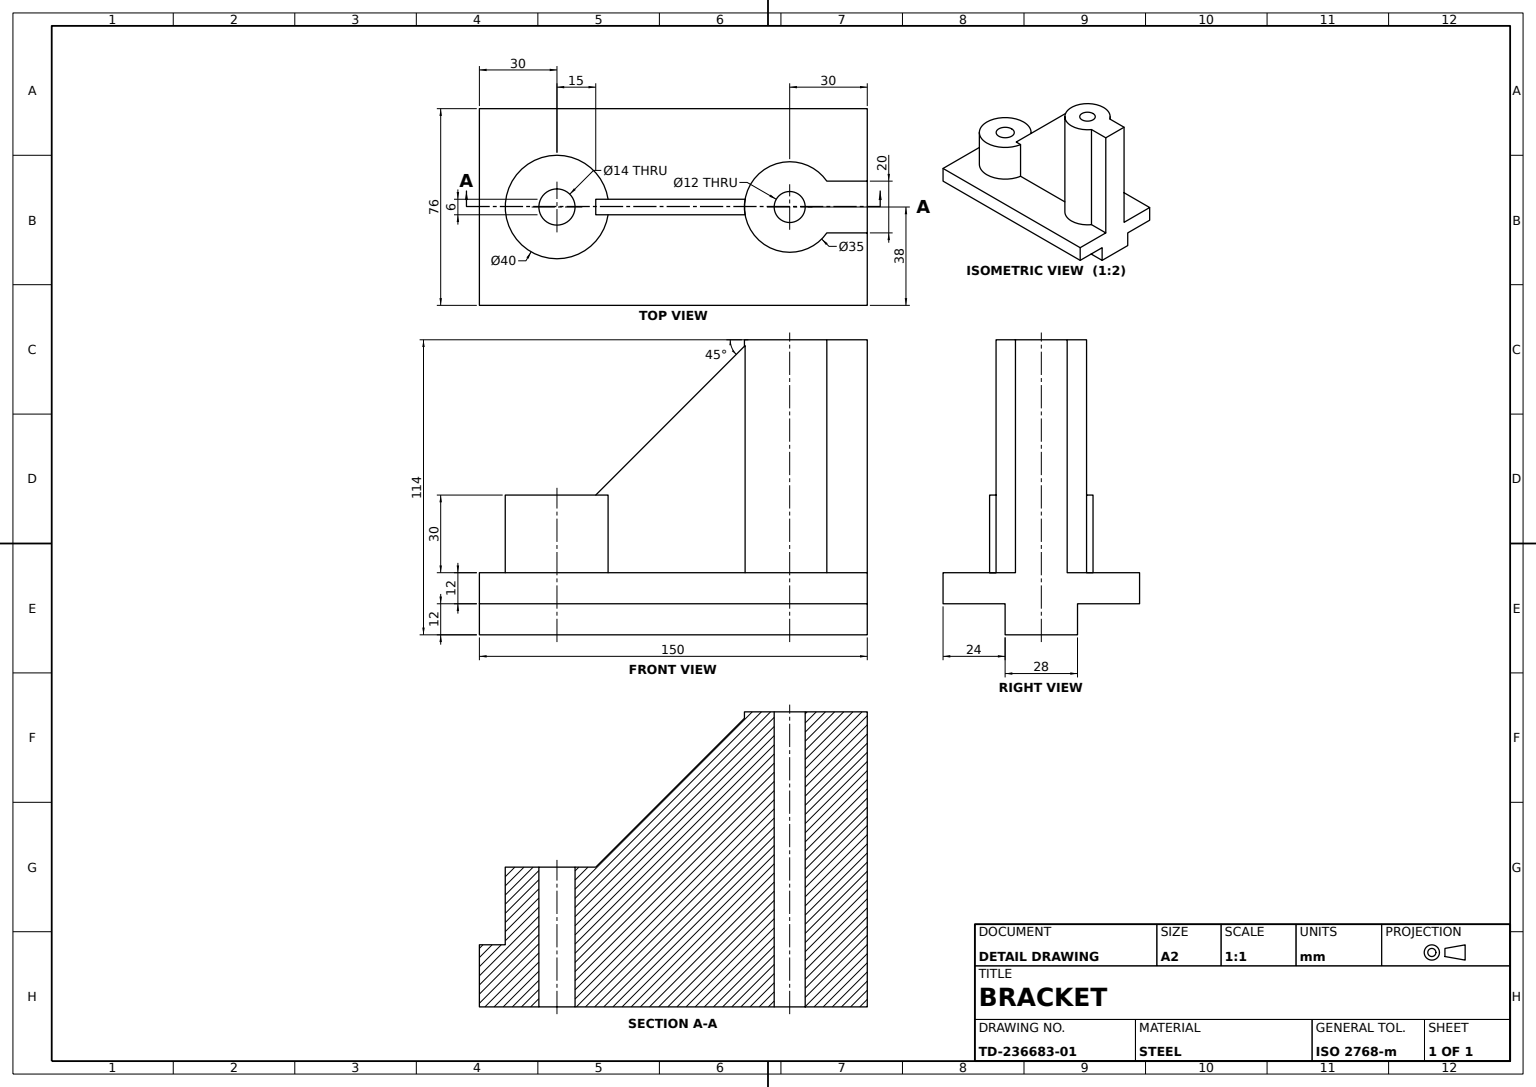
from build123d import *

# Parameters (mm, degrees)
BASE_PLATE_DEPTH          = 150
WEB_RIB_DEPTH             = 3
TALL_BOSS_PROFILE_R       = 17.5
TALL_BOSS_35_DEPTH        = 90
TALL_BOSS_BORE_PROFILE_R  = 6
TALL_BOSS_BORE_12_DEPTH   = 204.155113152
SHORT_BOSS_PROFILE_R      = 20
SHORT_BOSS_40_DEPTH       = 30
SHORT_BOSS_BORE_PROFILE_R = 7
SHORT_BOSS_BORE_14_DEPTH  = 179.538511252
SIDE_LUG_DEPTH            = 20


with BuildPart() as part:
    # Base Plate Profile → Base Plate (new body)
    with BuildSketch(Plane(origin=(0, 0, 0), x_dir=(0, 0, -1), z_dir=(1, 0, 0))):
        Polygon((0, 0), (0, 12), (76, 12), (76, 0), (52, 0), (52, -12), (24, -12), (24, 0), align=None)
    extrude(amount=BASE_PLATE_DEPTH)

    # Web Rib Profile → Web Rib (add, symmetric)
    with BuildSketch(Plane.XY.offset(-38)):
        Polygon((75, 12), (105, 12), (105, 102), (45, 42), (45, 12), align=None)
    extrude(amount=WEB_RIB_DEPTH, both=True)

    # Tall Boss Profile → Tall Boss Ø35 (add)
    with BuildSketch(Plane(origin=(0, 12, 0), x_dir=(1, 0, 0), z_dir=(0, 1, 0))):
        with Locations(Location((120, 38, 0), (0, 0, 170.129110394))):
            Circle(TALL_BOSS_PROFILE_R)
    extrude(amount=TALL_BOSS_35_DEPTH)

    # Tall Boss Bore Profile → Tall Boss Bore Ø12 (cut, through all)
    with BuildSketch(Plane(origin=(0, 102, 0), x_dir=(1, 0, 0), z_dir=(0, 1, 0))):
        with Locations(Location((120, 38, 0), (0, 0, 270))):
            Circle(TALL_BOSS_BORE_PROFILE_R)
    extrude(amount=-TALL_BOSS_BORE_12_DEPTH, mode=Mode.SUBTRACT)

    # Short Boss Profile → Short Boss Ø40 (add)
    with BuildSketch(Plane(origin=(0, 12, 0), x_dir=(1, 0, 0), z_dir=(0, 1, 0))):
        with Locations((30, 38)):
            Circle(SHORT_BOSS_PROFILE_R)
    extrude(amount=SHORT_BOSS_40_DEPTH)

    # Short Boss Bore Profile → Short Boss Bore Ø14 (cut, through all)
    with BuildSketch(Plane(origin=(0, 42, 0), x_dir=(1, 0, 0), z_dir=(0, 1, 0))):
        with Locations(Location((30, 38, 0), (0, 0, 270))):
            Circle(SHORT_BOSS_BORE_PROFILE_R)
    extrude(amount=-SHORT_BOSS_BORE_14_DEPTH, mode=Mode.SUBTRACT)

    # Side Lug Profile → Side Lug (add)
    with BuildSketch(Plane(origin=(150, 0, 0), x_dir=(0, 0, -1), z_dir=(1, 0, 0))):
        Polygon((38, 12), (28, 12), (28, 102), (48, 102), (48, 12), align=None)
    extrude(amount=-SIDE_LUG_DEPTH)


solid = part.part
